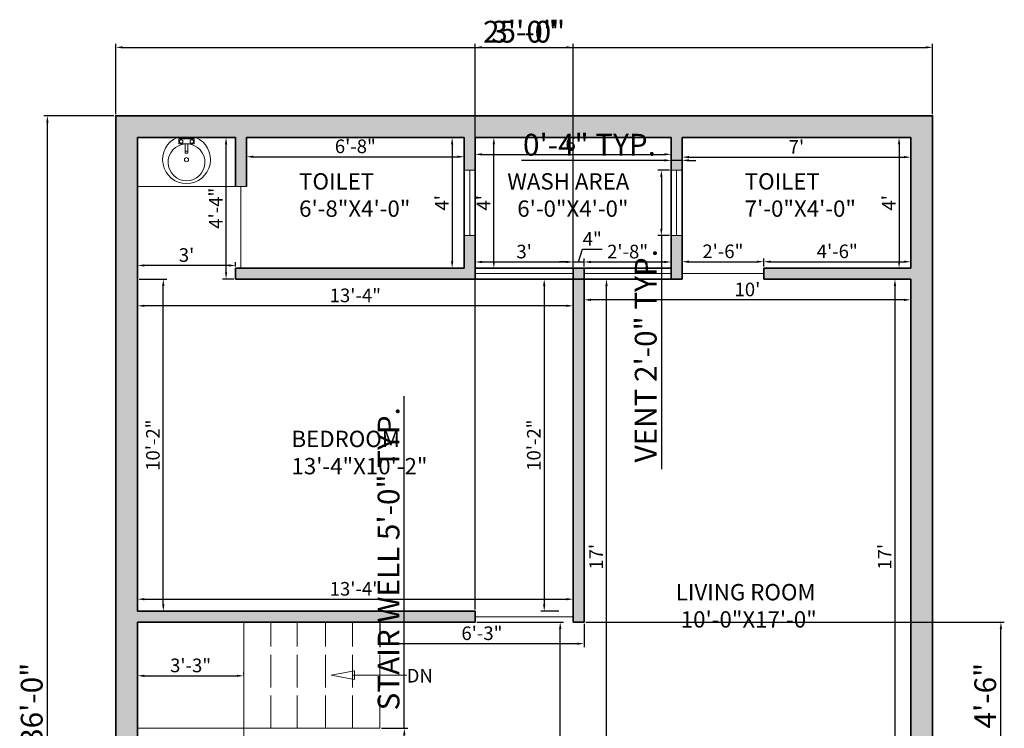
# Model space of a CAD drawing. Units: inches. Extents: x 3259 to 4981, y 1402 to 2026.
# Tile 11 of 11: x 4620 to 4981, y 1682 to 1942. Entities that reach past the tile are written whole.
import ezdxf

# ---------------------------------------------------------------- set-up
doc = ezdxf.new("R2010")
doc.units = ezdxf.units.IN
doc.linetypes.add('ACAD_ISO02W100', pattern=[15, 12, -3])
for name, color, linetype, lineweight in [('A-ANNO-DIMS', 2, 'Continuous', 13), ('A-ANNO-SYMB', 7, 'Continuous', 13), ('A-AREA-IDEN', 7, 'Continuous', 18), ('A-DOOR', 3, 'Continuous', 18), ('A-FLOR-CASE', 8, 'Continuous', 18), ('A-FLOR-FIXT', 9, 'Continuous', 18), ('A-FLOR-STRS', 7, 'Continuous', 18), ('A-FLOR-STRS-OVHD', 8, 'ACAD_ISO02W100', 13), ('A-GLAZ', 4, 'Continuous', 18), ('A-WALL', 7, 'Continuous', 35), ('A-WALL-PATT', 252, 'Continuous', 13)]:
    doc.layers.add(name, color=color, linetype=linetype, lineweight=lineweight)
doc.styles.get("Standard").update_dxf_attribs({"font": 'arial.ttf'})
doc.dimstyles.new('ISO-25', dxfattribs={"dimtxt": 8, "dimasz": 2.5, "dimexe": 1.25, "dimexo": 0.625, "dimtad": 1, "dimdec": 1, "dimlunit": 3, "dimtxsty": 'Standard', "dimcen": 2.5, "dimclrd": 4, "dimclre": 4, "dimclrt": 1, "dimadec": 0, "dimazin": 0, "dimtfac": 1, "dimtdec": 1, "dimtmove": 0, "dimatfit": 3, "dimfxl": 1, "dimarcsym": 0})

# ---------------------------------------------------------------- blocks, each defined once
blk = doc.blocks.new('M_BATH_BASIN_Basin - Oval_P')
at = {"color": 0, "linetype": 'ByBlock', "lineweight": -2}
blk.add_lwpolyline([(0, 89.5, -5.027337), (0, -89.5)], format="xyb", close=True, dxfattribs=at)
blk.add_lwpolyline([(63.2, 12, -30), (63.2, -12, -1.097889)], format="xyb", dxfattribs=at)
for points in [[(13.2, -76.2), (13.2, 76.2), (63.2, 76.2), (63.2, -76.2)], [(19.1, 50.8), (28.7, 67.3), (47.7, 67.3), (57.2, 50.8), (47.7, 34.3), (28.7, 34.3)]]:
    blk.add_lwpolyline(points, close=True, dxfattribs=at)
for points in [[(63.2, 12), (151.6, 12), (151.6, -12), (63.2, -12)], [(134.3, 12), (134.3, -12)], [(28.7, -34.3), (47.7, -34.3), (57.2, -50.8), (47.7, -67.3), (28.7, -67.3), (19.1, -50.8), (28.7, -34.3)]]:
    blk.add_lwpolyline(points, dxfattribs=at)
blk.add_circle((216.2, 0), 20.1, dxfattribs=at)
at = {"layer": 'Defpoints'}
for p in [(0, 234), (0, -234)]:
    blk.add_point(p, dxfattribs=at)
blk = doc.blocks.new('*D71')
at = {"layer": 'A-ANNO-DIMS', "color": 0, "lineweight": -2, "transparency": 16777216}
for p, q in [((4702.83, 1898.49), (4702.83, 1890.79)), ((4782.83, 1898.49), (4782.83, 1890.79)), ((4705.33, 1892.04), (4780.33, 1892.04))]:
    blk.add_line(p, q, dxfattribs=at)
at = {"layer": 'A-ANNO-DIMS', "color": 0, "transparency": 16777216}
for points in [[(4705.33, 1892.46), (4705.33, 1891.63), (4702.83, 1892.04)], [(4780.33, 1892.46), (4780.33, 1891.63), (4782.83, 1892.04)]]:
    blk.add_solid(points, dxfattribs=at)
at = {"layer": 'Defpoints', "color": 0, "transparency": 16777216}
for p in [(4702.83, 1899.12), (4782.83, 1899.12), (4782.83, 1892.04)]:
    blk.add_point(p, dxfattribs=at)
at = {"layer": 'A-ANNO-DIMS', "color": 0, "transparency": 16777216, "insert": (4742.83, 1895.22), "char_height": 5, "attachment_point": 5}
blk.add_mtext('6\'-8"', dxfattribs=at)
blk = doc.blocks.new('*D72')
at = {"layer": 'A-ANNO-DIMS', "color": 0, "lineweight": -2, "transparency": 16777216}
for p, q in [((4782.2, 1899.12), (4777.14, 1899.12)), ((4778.39, 1896.62), (4778.39, 1853.62)), ((4782.2, 1851.12), (4777.14, 1851.12))]:
    blk.add_line(p, q, dxfattribs=at)
at = {"layer": 'A-ANNO-DIMS', "color": 0, "transparency": 16777216}
for points in [[(4777.97, 1896.62), (4778.8, 1896.62), (4778.39, 1899.12)], [(4777.97, 1853.62), (4778.8, 1853.62), (4778.39, 1851.12)]]:
    blk.add_solid(points, dxfattribs=at)
at = {"layer": 'Defpoints', "color": 0, "transparency": 16777216}
for p in [(4782.83, 1899.12), (4778.39, 1851.12), (4782.83, 1851.12)]:
    blk.add_point(p, dxfattribs=at)
at = {"layer": 'A-ANNO-DIMS', "color": 0, "transparency": 16777216, "insert": (4775.26, 1875.12), "char_height": 5, "attachment_point": 5, "rotation": 90}
blk.add_mtext("4'", dxfattribs=at)
blk = doc.blocks.new('*D73')
at = {"layer": 'A-ANNO-DIMS', "color": 0, "lineweight": -2, "transparency": 16777216}
for p, q in [((4787.45, 1899.12), (4794.95, 1899.12)), ((4793.7, 1853.62), (4793.7, 1896.62)), ((4787.45, 1851.12), (4794.95, 1851.12))]:
    blk.add_line(p, q, dxfattribs=at)
at = {"layer": 'A-ANNO-DIMS', "color": 0, "transparency": 16777216}
for points in [[(4793.28, 1896.62), (4794.12, 1896.62), (4793.7, 1899.12)], [(4793.28, 1853.62), (4794.12, 1853.62), (4793.7, 1851.12)]]:
    blk.add_solid(points, dxfattribs=at)
at = {"layer": 'Defpoints', "color": 0, "transparency": 16777216}
for p in [(4786.83, 1899.12), (4793.7, 1899.12), (4786.83, 1851.12)]:
    blk.add_point(p, dxfattribs=at)
at = {"layer": 'A-ANNO-DIMS', "color": 0, "transparency": 16777216, "insert": (4790.57, 1875.12), "char_height": 5, "attachment_point": 5, "rotation": 90}
blk.add_mtext("4'", dxfattribs=at)
blk = doc.blocks.new('*D95')
at = {"layer": 'A-ANNO-DIMS', "color": 0, "lineweight": -2, "transparency": 16777216}
for p, q in [((4786.83, 1898.49), (4786.83, 1891.66)), ((4858.83, 1898.49), (4858.83, 1891.66)), ((4789.33, 1892.91), (4856.33, 1892.91))]:
    blk.add_line(p, q, dxfattribs=at)
at = {"layer": 'A-ANNO-DIMS', "color": 0, "transparency": 16777216}
for points in [[(4789.33, 1893.33), (4789.33, 1892.5), (4786.83, 1892.91)], [(4856.33, 1893.33), (4856.33, 1892.5), (4858.83, 1892.91)]]:
    blk.add_solid(points, dxfattribs=at)
at = {"layer": 'Defpoints', "color": 0, "transparency": 16777216}
for p in [(4786.83, 1899.12), (4858.83, 1899.12), (4858.83, 1892.91)]:
    blk.add_point(p, dxfattribs=at)
at = {"layer": 'A-ANNO-DIMS', "color": 0, "transparency": 16777216, "insert": (4822.83, 1896.09), "char_height": 5, "attachment_point": 5}
blk.add_mtext("6'", dxfattribs=at)
blk = doc.blocks.new('*D96')
at = {"layer": 'A-ANNO-DIMS', "color": 0, "lineweight": -2, "transparency": 16777216}
for p, q in [((4862.83, 1898.49), (4862.83, 1890.65)), ((4946.83, 1898.49), (4946.83, 1890.65)), ((4865.33, 1891.9), (4944.33, 1891.9))]:
    blk.add_line(p, q, dxfattribs=at)
at = {"layer": 'A-ANNO-DIMS', "color": 0, "transparency": 16777216}
for points in [[(4865.33, 1892.31), (4865.33, 1891.48), (4862.83, 1891.9)], [(4944.33, 1892.31), (4944.33, 1891.48), (4946.83, 1891.9)]]:
    blk.add_solid(points, dxfattribs=at)
at = {"layer": 'Defpoints', "color": 0, "transparency": 16777216}
for p in [(4862.83, 1899.12), (4946.83, 1899.12), (4946.83, 1891.9)]:
    blk.add_point(p, dxfattribs=at)
at = {"layer": 'A-ANNO-DIMS', "color": 0, "transparency": 16777216, "insert": (4904.83, 1895.02), "char_height": 5, "attachment_point": 5}
blk.add_mtext("7'", dxfattribs=at)
blk = doc.blocks.new('*D97')
at = {"layer": 'A-ANNO-DIMS', "color": 0, "lineweight": -2, "transparency": 16777216}
for p, q in [((4946.2, 1899.12), (4941.29, 1899.12)), ((4942.54, 1896.62), (4942.54, 1853.62)), ((4946.2, 1851.12), (4941.29, 1851.12))]:
    blk.add_line(p, q, dxfattribs=at)
at = {"layer": 'A-ANNO-DIMS', "color": 0, "transparency": 16777216}
for points in [[(4942.13, 1896.62), (4942.96, 1896.62), (4942.54, 1899.12)], [(4942.13, 1853.62), (4942.96, 1853.62), (4942.54, 1851.12)]]:
    blk.add_solid(points, dxfattribs=at)
at = {"layer": 'Defpoints', "color": 0, "transparency": 16777216}
for p in [(4946.83, 1899.12), (4942.54, 1851.12), (4946.83, 1851.12)]:
    blk.add_point(p, dxfattribs=at)
at = {"layer": 'A-ANNO-DIMS', "color": 0, "transparency": 16777216, "insert": (4939.42, 1875.12), "char_height": 5, "attachment_point": 5, "rotation": 90}
blk.add_mtext("4'", dxfattribs=at)
blk = doc.blocks.new('*D86')
at = {"layer": 'A-ANNO-DIMS', "color": 0, "lineweight": -2, "transparency": 16777216}
for p, q in [((4787.45, 1721.12), (4819.32, 1721.12)), ((4818.07, 1585.62), (4818.07, 1718.62)), ((4822.2, 1583.12), (4816.82, 1583.12))]:
    blk.add_line(p, q, dxfattribs=at)
at = {"layer": 'A-ANNO-DIMS', "color": 0, "transparency": 16777216}
for points in [[(4817.66, 1718.62), (4818.49, 1718.62), (4818.07, 1721.12)], [(4817.66, 1585.62), (4818.49, 1585.62), (4818.07, 1583.12)]]:
    blk.add_solid(points, dxfattribs=at)
at = {"layer": 'Defpoints', "color": 0, "transparency": 16777216}
for p in [(4786.83, 1721.12), (4818.07, 1721.12), (4822.83, 1583.12)]:
    blk.add_point(p, dxfattribs=at)
at = {"layer": 'A-ANNO-DIMS', "color": 0, "transparency": 16777216, "insert": (4814.9, 1652.12), "char_height": 5, "attachment_point": 5, "rotation": 90}
blk.add_mtext('11\'-6"', dxfattribs=at)
blk = doc.blocks.new('*D88')
at = {"layer": 'A-ANNO-DIMS', "color": 0, "lineweight": -2, "transparency": 16777216}
for p, q in [((4827.45, 1847.12), (4836.33, 1847.12)), ((4835.08, 1645.62), (4835.08, 1844.62)), ((4827.45, 1643.12), (4836.33, 1643.12))]:
    blk.add_line(p, q, dxfattribs=at)
at = {"layer": 'A-ANNO-DIMS', "color": 0, "transparency": 16777216}
for points in [[(4834.66, 1844.62), (4835.49, 1844.62), (4835.08, 1847.12)], [(4834.66, 1645.62), (4835.49, 1645.62), (4835.08, 1643.12)]]:
    blk.add_solid(points, dxfattribs=at)
at = {"layer": 'Defpoints', "color": 0, "transparency": 16777216}
for p in [(4826.83, 1847.12), (4835.08, 1847.12), (4826.83, 1643.12)]:
    blk.add_point(p, dxfattribs=at)
at = {"layer": 'A-ANNO-DIMS', "color": 0, "transparency": 16777216, "insert": (4831.94, 1745.12), "char_height": 5, "attachment_point": 5, "rotation": 90}
blk.add_mtext("17'", dxfattribs=at)
blk = doc.blocks.new('*D89')
at = {"layer": 'A-ANNO-DIMS', "color": 0, "lineweight": -2, "transparency": 16777216}
for p, q in [((4662.83, 1702.02), (4662.83, 1702.65)), ((4665.33, 1701.4), (4699.33, 1701.4)), ((4701.83, 1702.02), (4701.83, 1702.65))]:
    blk.add_line(p, q, dxfattribs=at)
at = {"layer": 'A-ANNO-DIMS', "color": 0, "transparency": 16777216}
for points in [[(4665.33, 1701.81), (4665.33, 1700.98), (4662.83, 1701.4)], [(4699.33, 1701.81), (4699.33, 1700.98), (4701.83, 1701.4)]]:
    blk.add_solid(points, dxfattribs=at)
at = {"layer": 'Defpoints', "color": 0, "transparency": 16777216}
for p in [(4662.83, 1701.4), (4701.83, 1701.4), (4701.83, 1701.4)]:
    blk.add_point(p, dxfattribs=at)
at = {"layer": 'A-ANNO-DIMS', "color": 0, "transparency": 16777216, "insert": (4682.33, 1704.57), "char_height": 5, "attachment_point": 5}
blk.add_mtext('3\'-3"', dxfattribs=at)
blk = doc.blocks.new('*D98')
at = {"layer": 'A-ANNO-DIMS', "color": 0, "lineweight": -2, "transparency": 16777216}
for p, q in [((4826.83, 1848.49), (4826.83, 1838.23)), ((4946.83, 1846.49), (4946.83, 1838.23)), ((4944.33, 1839.48), (4829.33, 1839.48))]:
    blk.add_line(p, q, dxfattribs=at)
at = {"layer": 'A-ANNO-DIMS', "color": 0, "transparency": 16777216}
for points in [[(4829.33, 1839.9), (4829.33, 1839.07), (4826.83, 1839.48)], [(4944.33, 1839.9), (4944.33, 1839.07), (4946.83, 1839.48)]]:
    blk.add_solid(points, dxfattribs=at)
at = {"layer": 'Defpoints', "color": 0, "transparency": 16777216}
for p in [(4826.83, 1849.12), (4946.83, 1847.12), (4826.83, 1839.48)]:
    blk.add_point(p, dxfattribs=at)
at = {"layer": 'A-ANNO-DIMS', "color": 0, "transparency": 16777216, "insert": (4886.83, 1842.66), "char_height": 5, "attachment_point": 5}
blk.add_mtext("10'", dxfattribs=at)
blk = doc.blocks.new('*D99')
at = {"layer": 'A-ANNO-DIMS', "color": 0, "lineweight": -2, "transparency": 16777216}
for p, q in [((4946.2, 1847.12), (4939.77, 1847.12)), ((4941.02, 1844.62), (4941.02, 1645.62)), ((4946.2, 1643.12), (4939.77, 1643.12))]:
    blk.add_line(p, q, dxfattribs=at)
at = {"layer": 'A-ANNO-DIMS', "color": 0, "transparency": 16777216}
for points in [[(4940.61, 1844.62), (4941.44, 1844.62), (4941.02, 1847.12)], [(4940.61, 1645.62), (4941.44, 1645.62), (4941.02, 1643.12)]]:
    blk.add_solid(points, dxfattribs=at)
at = {"layer": 'Defpoints', "color": 0, "transparency": 16777216}
for p in [(4946.83, 1847.12), (4941.02, 1643.12), (4946.83, 1643.12)]:
    blk.add_point(p, dxfattribs=at)
at = {"layer": 'A-ANNO-DIMS', "color": 0, "transparency": 16777216, "insert": (4937.89, 1745.12), "char_height": 5, "attachment_point": 5, "rotation": 90}
blk.add_mtext("17'", dxfattribs=at)
blk = doc.blocks.new('*D100')
at = {"layer": 'A-ANNO-DIMS', "color": 0, "lineweight": -2, "transparency": 16777216}
for p, q in [((4662.83, 1846.49), (4662.83, 1836.05)), ((4822.83, 1846.49), (4822.83, 1836.05)), ((4820.33, 1837.3), (4665.33, 1837.3))]:
    blk.add_line(p, q, dxfattribs=at)
at = {"layer": 'A-ANNO-DIMS', "color": 0, "transparency": 16777216}
for points in [[(4665.33, 1837.71), (4665.33, 1836.88), (4662.83, 1837.3)], [(4820.33, 1837.71), (4820.33, 1836.88), (4822.83, 1837.3)]]:
    blk.add_solid(points, dxfattribs=at)
at = {"layer": 'Defpoints', "color": 0, "transparency": 16777216}
for p in [(4662.83, 1847.12), (4822.83, 1847.12), (4662.83, 1837.3)]:
    blk.add_point(p, dxfattribs=at)
at = {"layer": 'A-ANNO-DIMS', "color": 0, "transparency": 16777216, "insert": (4742.83, 1840.48), "char_height": 5, "attachment_point": 5}
blk.add_mtext('13\'-4"', dxfattribs=at)
blk = doc.blocks.new('*D101')
at = {"layer": 'A-ANNO-DIMS', "color": 0, "lineweight": -2, "transparency": 16777216}
for p, q in [((4662.83, 1725.74), (4662.83, 1730.78)), ((4665.33, 1729.53), (4820.33, 1729.53)), ((4822.83, 1725.74), (4822.83, 1730.78))]:
    blk.add_line(p, q, dxfattribs=at)
at = {"layer": 'A-ANNO-DIMS', "color": 0, "transparency": 16777216}
for points in [[(4665.33, 1729.95), (4665.33, 1729.12), (4662.83, 1729.53)], [(4820.33, 1729.95), (4820.33, 1729.12), (4822.83, 1729.53)]]:
    blk.add_solid(points, dxfattribs=at)
at = {"layer": 'Defpoints', "color": 0, "transparency": 16777216}
for p in [(4822.83, 1729.53), (4662.83, 1725.12), (4822.83, 1725.12)]:
    blk.add_point(p, dxfattribs=at)
at = {"layer": 'A-ANNO-DIMS', "color": 0, "transparency": 16777216, "insert": (4742.83, 1732.71), "char_height": 5, "attachment_point": 5}
blk.add_mtext('13\'-4"', dxfattribs=at)
blk = doc.blocks.new('*D102')
at = {"layer": 'A-ANNO-DIMS', "color": 0, "lineweight": -2, "transparency": 16777216}
for p, q in [((4663.45, 1847.12), (4673.56, 1847.12)), ((4672.31, 1727.62), (4672.31, 1844.62)), ((4663.45, 1725.12), (4673.56, 1725.12))]:
    blk.add_line(p, q, dxfattribs=at)
at = {"layer": 'A-ANNO-DIMS', "color": 0, "transparency": 16777216}
for points in [[(4671.9, 1844.62), (4672.73, 1844.62), (4672.31, 1847.12)], [(4671.9, 1727.62), (4672.73, 1727.62), (4672.31, 1725.12)]]:
    blk.add_solid(points, dxfattribs=at)
at = {"layer": 'Defpoints', "color": 0, "transparency": 16777216}
for p in [(4662.83, 1847.12), (4672.31, 1847.12), (4662.83, 1725.12)]:
    blk.add_point(p, dxfattribs=at)
at = {"layer": 'A-ANNO-DIMS', "color": 0, "transparency": 16777216, "insert": (4669.13, 1786.12), "char_height": 5, "attachment_point": 5, "rotation": 90}
blk.add_mtext('10\'-2"', dxfattribs=at)
blk = doc.blocks.new('*D103')
at = {"layer": 'A-ANNO-DIMS', "color": 0, "lineweight": -2, "transparency": 16777216}
for p, q in [((4817.52, 1847.12), (4810.96, 1847.12)), ((4812.21, 1844.62), (4812.21, 1727.62)), ((4817.52, 1725.12), (4810.96, 1725.12))]:
    blk.add_line(p, q, dxfattribs=at)
at = {"layer": 'A-ANNO-DIMS', "color": 0, "transparency": 16777216}
for points in [[(4811.79, 1844.62), (4812.62, 1844.62), (4812.21, 1847.12)], [(4811.79, 1727.62), (4812.62, 1727.62), (4812.21, 1725.12)]]:
    blk.add_solid(points, dxfattribs=at)
at = {"layer": 'Defpoints', "color": 0, "transparency": 16777216}
for p in [(4818.15, 1847.12), (4812.21, 1725.12), (4818.15, 1725.12)]:
    blk.add_point(p, dxfattribs=at)
at = {"layer": 'A-ANNO-DIMS', "color": 0, "transparency": 16777216, "insert": (4809.03, 1786.12), "char_height": 5, "attachment_point": 5, "rotation": 90}
blk.add_mtext('10\'-2"', dxfattribs=at)
blk = doc.blocks.new('*D104')
at = {"layer": 'A-ANNO-DIMS', "color": 0, "lineweight": -2, "transparency": 16777216}
for p, q in [((4662.83, 1851.74), (4662.83, 1853.36)), ((4696.33, 1852.11), (4665.33, 1852.11)), ((4698.83, 1851.74), (4698.83, 1853.36))]:
    blk.add_line(p, q, dxfattribs=at)
at = {"layer": 'A-ANNO-DIMS', "color": 0, "transparency": 16777216}
for points in [[(4665.33, 1852.52), (4665.33, 1851.69), (4662.83, 1852.11)], [(4696.33, 1852.52), (4696.33, 1851.69), (4698.83, 1852.11)]]:
    blk.add_solid(points, dxfattribs=at)
at = {"layer": 'Defpoints', "color": 0, "transparency": 16777216}
for p in [(4662.83, 1852.11), (4662.83, 1851.12), (4698.83, 1851.12)]:
    blk.add_point(p, dxfattribs=at)
at = {"layer": 'A-ANNO-DIMS', "color": 0, "transparency": 16777216, "insert": (4680.83, 1855.29), "char_height": 5, "attachment_point": 5}
blk.add_mtext("3'", dxfattribs=at)
blk = doc.blocks.new('*D105')
at = {"layer": 'A-ANNO-DIMS', "color": 0, "lineweight": -2, "transparency": 16777216}
for p, q in [((4698.2, 1899.12), (4694.11, 1899.12)), ((4695.36, 1849.62), (4695.36, 1896.62)), ((4698.2, 1847.12), (4694.11, 1847.12))]:
    blk.add_line(p, q, dxfattribs=at)
at = {"layer": 'A-ANNO-DIMS', "color": 0, "transparency": 16777216}
for points in [[(4694.95, 1896.62), (4695.78, 1896.62), (4695.36, 1899.12)], [(4694.95, 1849.62), (4695.78, 1849.62), (4695.36, 1847.12)]]:
    blk.add_solid(points, dxfattribs=at)
at = {"layer": 'Defpoints', "color": 0, "transparency": 16777216}
for p in [(4695.36, 1899.12), (4698.83, 1899.12), (4698.83, 1847.12)]:
    blk.add_point(p, dxfattribs=at)
at = {"layer": 'A-ANNO-DIMS', "color": 0, "transparency": 16777216, "insert": (4692.24, 1873.12), "char_height": 5, "attachment_point": 5, "rotation": 90}
blk.add_mtext('4\'-4"', dxfattribs=at)
blk = doc.blocks.new('*D106')
at = {"layer": 'A-ANNO-DIMS', "color": 0, "lineweight": -2, "transparency": 16777216}
for p, q in [((4751.83, 1720.49), (4751.83, 1711.96)), ((4826.83, 1720.49), (4826.83, 1711.96)), ((4754.33, 1713.21), (4824.33, 1713.21))]:
    blk.add_line(p, q, dxfattribs=at)
at = {"layer": 'A-ANNO-DIMS', "color": 0, "transparency": 16777216}
for points in [[(4754.33, 1713.63), (4754.33, 1712.8), (4751.83, 1713.21)], [(4824.33, 1713.63), (4824.33, 1712.8), (4826.83, 1713.21)]]:
    blk.add_solid(points, dxfattribs=at)
at = {"layer": 'Defpoints', "color": 0, "transparency": 16777216}
for p in [(4751.83, 1721.12), (4826.83, 1721.12), (4826.83, 1713.21)]:
    blk.add_point(p, dxfattribs=at)
at = {"layer": 'A-ANNO-DIMS', "color": 0, "transparency": 16777216, "insert": (4789.33, 1716.39), "char_height": 5, "attachment_point": 5}
blk.add_mtext('6\'-3"', dxfattribs=at)
blk = doc.blocks.new('*D127')
at = {"layer": 'A-ANNO-DIMS', "color": 0, "lineweight": -2, "transparency": 16777216}
for p, q in [((4786.83, 1851.74), (4786.83, 1854.64)), ((4789.33, 1853.39), (4820.33, 1853.39)), ((4822.83, 1851.74), (4822.83, 1854.64))]:
    blk.add_line(p, q, dxfattribs=at)
at = {"layer": 'A-ANNO-DIMS', "color": 0, "transparency": 16777216}
for points in [[(4789.33, 1853.81), (4789.33, 1852.97), (4786.83, 1853.39)], [(4820.33, 1853.81), (4820.33, 1852.97), (4822.83, 1853.39)]]:
    blk.add_solid(points, dxfattribs=at)
at = {"layer": 'Defpoints', "color": 0, "transparency": 16777216}
for p in [(4822.83, 1853.39), (4786.83, 1851.12), (4822.83, 1851.12)]:
    blk.add_point(p, dxfattribs=at)
at = {"layer": 'A-ANNO-DIMS', "color": 0, "transparency": 16777216, "insert": (4804.83, 1856.57), "char_height": 5, "attachment_point": 5}
blk.add_mtext("3'", dxfattribs=at)
blk = doc.blocks.new('*D128')
at = {"layer": 'A-ANNO-DIMS', "color": 0, "lineweight": -2, "transparency": 16777216}
for p, q in [((4824.83, 1853.39), (4826.24, 1858.08)), ((4826.24, 1858.08), (4833.43, 1858.08)), ((4820.33, 1853.39), (4817.83, 1853.39)), ((4822.83, 1851.74), (4822.83, 1854.64)), ((4822.83, 1853.39), (4826.83, 1853.39)), ((4822.83, 1853.39), (4826.83, 1853.39)), ((4826.83, 1851.74), (4826.83, 1854.64)), ((4829.33, 1853.39), (4831.83, 1853.39))]:
    blk.add_line(p, q, dxfattribs=at)
at = {"layer": 'A-ANNO-DIMS', "color": 0, "transparency": 16777216}
for points in [[(4820.33, 1853.81), (4820.33, 1852.97), (4822.83, 1853.39)], [(4829.33, 1853.81), (4829.33, 1852.97), (4826.83, 1853.39)]]:
    blk.add_solid(points, dxfattribs=at)
at = {"layer": 'Defpoints', "color": 0, "transparency": 16777216}
for p in [(4826.83, 1853.39), (4822.83, 1851.12), (4826.83, 1851.12)]:
    blk.add_point(p, dxfattribs=at)
at = {"layer": 'A-ANNO-DIMS', "color": 0, "transparency": 16777216, "insert": (4829.84, 1861.2), "char_height": 5, "attachment_point": 5}
blk.add_mtext('4"', dxfattribs=at)
blk = doc.blocks.new('*D129')
at = {"layer": 'A-ANNO-DIMS', "color": 0, "lineweight": -2, "transparency": 16777216}
for p, q in [((4826.83, 1851.74), (4826.83, 1854.64)), ((4829.33, 1853.39), (4856.33, 1853.39)), ((4858.83, 1851.74), (4858.83, 1854.64))]:
    blk.add_line(p, q, dxfattribs=at)
at = {"layer": 'A-ANNO-DIMS', "color": 0, "transparency": 16777216}
for points in [[(4829.33, 1853.81), (4829.33, 1852.97), (4826.83, 1853.39)], [(4856.33, 1853.81), (4856.33, 1852.97), (4858.83, 1853.39)]]:
    blk.add_solid(points, dxfattribs=at)
at = {"layer": 'Defpoints', "color": 0, "transparency": 16777216}
for p in [(4858.83, 1853.39), (4826.83, 1851.12), (4858.83, 1851.12)]:
    blk.add_point(p, dxfattribs=at)
at = {"layer": 'A-ANNO-DIMS', "color": 0, "transparency": 16777216, "insert": (4842.83, 1856.57), "char_height": 5, "attachment_point": 5}
blk.add_mtext('2\'-8"', dxfattribs=at)
blk = doc.blocks.new('*D130')
at = {"layer": 'A-ANNO-DIMS', "color": 0, "lineweight": -2, "transparency": 16777216}
for p, q in [((4862.83, 1854.02), (4862.83, 1854.73)), ((4865.33, 1853.48), (4890.33, 1853.48)), ((4892.83, 1851.74), (4892.83, 1854.73))]:
    blk.add_line(p, q, dxfattribs=at)
at = {"layer": 'A-ANNO-DIMS', "color": 0, "transparency": 16777216}
for points in [[(4865.33, 1853.9), (4865.33, 1853.07), (4862.83, 1853.48)], [(4890.33, 1853.9), (4890.33, 1853.07), (4892.83, 1853.48)]]:
    blk.add_solid(points, dxfattribs=at)
at = {"layer": 'Defpoints', "color": 0, "transparency": 16777216}
for p in [(4862.83, 1853.39), (4892.83, 1853.48), (4892.83, 1851.12)]:
    blk.add_point(p, dxfattribs=at)
at = {"layer": 'A-ANNO-DIMS', "color": 0, "transparency": 16777216, "insert": (4877.83, 1856.66), "char_height": 5, "attachment_point": 5}
blk.add_mtext('2\'-6"', dxfattribs=at)
blk = doc.blocks.new('*D131')
at = {"layer": 'A-ANNO-DIMS', "color": 0, "lineweight": -2, "transparency": 16777216}
for p, q in [((4892.83, 1851.74), (4892.83, 1854.73)), ((4895.33, 1853.48), (4944.33, 1853.48)), ((4946.83, 1854.11), (4946.83, 1854.73))]:
    blk.add_line(p, q, dxfattribs=at)
at = {"layer": 'A-ANNO-DIMS', "color": 0, "transparency": 16777216}
for points in [[(4895.33, 1853.9), (4895.33, 1853.07), (4892.83, 1853.48)], [(4944.33, 1853.9), (4944.33, 1853.07), (4946.83, 1853.48)]]:
    blk.add_solid(points, dxfattribs=at)
at = {"layer": 'Defpoints', "color": 0, "transparency": 16777216}
for p in [(4946.83, 1853.48), (4946.83, 1853.48), (4892.83, 1851.12)]:
    blk.add_point(p, dxfattribs=at)
at = {"layer": 'A-ANNO-DIMS', "color": 0, "transparency": 16777216, "insert": (4919.83, 1856.66), "char_height": 5, "attachment_point": 5}
blk.add_mtext('4\'-6"', dxfattribs=at)
blk = doc.blocks.new('VENT-24x4')
for p, q in [((0, 24), (4, 24)), ((2, 24), (2, 0)), ((0, 0), (4, 0))]:
    blk.add_line(p, q)
blk = doc.blocks.new('STAIR-DIRECTION')
blk.add_line((7.93, 1.55), (27.85, 1.55))
blk.add_lwpolyline([(0, 1.55), (8.64, 3.11), (8.64, 0)], close=True)
blk = doc.blocks.new('*D146')
at = {"layer": 'A-ANNO-DIMS', "color": 4, "lineweight": -2, "transparency": 16777216}
for p, q in [((4858.2, 1887.12), (4853.98, 1887.12)), ((4855.23, 1884.62), (4855.23, 1865.62)), ((4858.2, 1863.12), (4853.98, 1863.12)), ((4855.23, 1863.12), (4855.23, 1777.28))]:
    blk.add_line(p, q, dxfattribs=at)
at = {"layer": 'A-ANNO-DIMS', "color": 4, "transparency": 16777216}
for points in [[(4854.81, 1884.62), (4855.65, 1884.62), (4855.23, 1887.12)], [(4854.81, 1865.62), (4855.65, 1865.62), (4855.23, 1863.12)]]:
    blk.add_solid(points, dxfattribs=at)
at = {"layer": 'Defpoints', "color": 0, "transparency": 16777216}
for p in [(4858.83, 1887.12), (4855.23, 1863.12), (4858.83, 1863.12)]:
    blk.add_point(p, dxfattribs=at)
at = {"layer": 'A-ANNO-DIMS', "color": 1, "transparency": 16777216, "insert": (4850.52, 1818.95), "char_height": 8, "attachment_point": 5, "rotation": 90}
blk.add_mtext('VENT 2\'-0" TYP.', dxfattribs=at)
blk = doc.blocks.new('*D147')
at = {"layer": 'A-ANNO-DIMS', "color": 4, "lineweight": -2, "transparency": 16777216}
for p, q in [((4858.83, 1887.74), (4858.83, 1891.97)), ((4862.83, 1887.74), (4862.83, 1891.97)), ((4856.33, 1890.72), (4803.82, 1890.72)), ((4862.83, 1890.72), (4858.83, 1890.72)), ((4865.33, 1890.72), (4867.83, 1890.72))]:
    blk.add_line(p, q, dxfattribs=at)
at = {"layer": 'A-ANNO-DIMS', "color": 4, "transparency": 16777216}
for points in [[(4856.33, 1891.13), (4856.33, 1890.3), (4858.83, 1890.72)], [(4865.33, 1891.13), (4865.33, 1890.3), (4862.83, 1890.72)]]:
    blk.add_solid(points, dxfattribs=at)
at = {"layer": 'Defpoints', "color": 0, "transparency": 16777216}
for p in [(4858.83, 1890.72), (4858.83, 1887.12), (4862.83, 1887.12)]:
    blk.add_point(p, dxfattribs=at)
at = {"layer": 'A-ANNO-DIMS', "color": 1, "transparency": 16777216, "insert": (4828.82, 1895.43), "char_height": 8, "attachment_point": 5}
blk.add_mtext('0\'-4" TYP.', dxfattribs=at)
blk = doc.blocks.new('*D154')
at = {"layer": 'A-ANNO-DIMS', "color": 4, "lineweight": -2, "transparency": 16777216}
for p, q in [((4760.83, 1682.12), (4760.83, 1804.15)), ((4752.45, 1682.12), (4762.08, 1682.12)), ((4760.83, 1624.62), (4760.83, 1679.62)), ((4752.45, 1622.12), (4762.08, 1622.12))]:
    blk.add_line(p, q, dxfattribs=at)
at = {"layer": 'A-ANNO-DIMS', "color": 4, "transparency": 16777216}
for points in [[(4760.41, 1679.62), (4761.25, 1679.62), (4760.83, 1682.12)], [(4760.41, 1624.62), (4761.25, 1624.62), (4760.83, 1622.12)]]:
    blk.add_solid(points, dxfattribs=at)
at = {"layer": 'Defpoints', "color": 0, "transparency": 16777216}
for p in [(4751.83, 1682.12), (4760.83, 1682.12), (4751.83, 1622.12)]:
    blk.add_point(p, dxfattribs=at)
at = {"layer": 'A-ANNO-DIMS', "color": 1, "transparency": 16777216, "insert": (4756.07, 1744.38), "char_height": 8, "attachment_point": 5, "rotation": 90}
blk.add_mtext('STAIR WELL 5\'-0" TYP.', dxfattribs=at)
blk = doc.blocks.new('*D188')
at = {"layer": 'A-ANNO-DIMS', "color": 4, "lineweight": -2, "transparency": 16777216}
for p, q in [((4654.83, 1907.74), (4654.83, 1933.47)), ((4657.33, 1932.22), (4952.33, 1932.22)), ((4954.83, 1907.74), (4954.83, 1933.47))]:
    blk.add_line(p, q, dxfattribs=at)
at = {"layer": 'A-ANNO-DIMS', "color": 4, "transparency": 16777216}
for points in [[(4657.33, 1932.63), (4657.33, 1931.8), (4654.83, 1932.22)], [(4952.33, 1932.63), (4952.33, 1931.8), (4954.83, 1932.22)]]:
    blk.add_solid(points, dxfattribs=at)
at = {"layer": 'Defpoints', "color": 0, "transparency": 16777216}
for p in [(4954.83, 1932.22), (4654.83, 1907.12), (4954.83, 1907.12)]:
    blk.add_point(p, dxfattribs=at)
at = {"layer": 'A-ANNO-DIMS', "color": 1, "transparency": 16777216, "insert": (4804.83, 1936.93), "char_height": 8, "attachment_point": 5}
blk.add_mtext('25\'-0"', dxfattribs=at)
blk = doc.blocks.new('*D189')
at = {"layer": 'A-ANNO-DIMS', "color": 4, "lineweight": -2, "transparency": 16777216}
for p, q in [((4654.2, 1907.12), (4628.48, 1907.12)), ((4629.73, 1477.62), (4629.73, 1904.62)), ((4654.2, 1475.12), (4628.48, 1475.12))]:
    blk.add_line(p, q, dxfattribs=at)
at = {"layer": 'A-ANNO-DIMS', "color": 4, "transparency": 16777216}
for points in [[(4629.31, 1904.62), (4630.15, 1904.62), (4629.73, 1907.12)], [(4629.31, 1477.62), (4630.15, 1477.62), (4629.73, 1475.12)]]:
    blk.add_solid(points, dxfattribs=at)
at = {"layer": 'Defpoints', "color": 0, "transparency": 16777216}
for p in [(4629.73, 1907.12), (4654.83, 1907.12), (4654.83, 1475.12)]:
    blk.add_point(p, dxfattribs=at)
at = {"layer": 'A-ANNO-DIMS', "color": 1, "transparency": 16777216, "insert": (4625.02, 1691.12), "char_height": 8, "attachment_point": 5, "rotation": 90}
blk.add_mtext('36\'-0"', dxfattribs=at)
blk = doc.blocks.new('*D196')
at = {"layer": 'A-ANNO-DIMS', "color": 4, "lineweight": -2, "transparency": 16777216}
for p, q in [((4786.83, 1725.74), (4786.83, 1933.47)), ((4789.33, 1932.22), (4820.33, 1932.22)), ((4822.83, 1723.74), (4822.83, 1933.47))]:
    blk.add_line(p, q, dxfattribs=at)
at = {"layer": 'A-ANNO-DIMS', "color": 4, "transparency": 16777216}
for points in [[(4789.33, 1932.63), (4789.33, 1931.8), (4786.83, 1932.22)], [(4820.33, 1932.63), (4820.33, 1931.8), (4822.83, 1932.22)]]:
    blk.add_solid(points, dxfattribs=at)
at = {"layer": 'Defpoints', "color": 0, "transparency": 16777216}
for p in [(4822.83, 1932.22), (4786.83, 1725.12), (4822.83, 1723.12)]:
    blk.add_point(p, dxfattribs=at)
at = {"layer": 'A-ANNO-DIMS', "color": 1, "transparency": 16777216, "insert": (4804.83, 1936.93), "char_height": 8, "attachment_point": 5}
blk.add_mtext('3\'-0"', dxfattribs=at)
blk = doc.blocks.new('*D197')
at = {"layer": 'A-ANNO-DIMS', "color": 4, "lineweight": -2, "transparency": 16777216}
for p, q in [((4827.45, 1721.12), (4981.18, 1721.12)), ((4979.93, 1669.62), (4979.93, 1718.62)), ((4827.45, 1667.12), (4981.18, 1667.12))]:
    blk.add_line(p, q, dxfattribs=at)
at = {"layer": 'A-ANNO-DIMS', "color": 4, "transparency": 16777216}
for points in [[(4979.51, 1718.62), (4980.35, 1718.62), (4979.93, 1721.12)], [(4979.51, 1669.62), (4980.35, 1669.62), (4979.93, 1667.12)]]:
    blk.add_solid(points, dxfattribs=at)
at = {"layer": 'Defpoints', "color": 0, "transparency": 16777216}
for p in [(4826.83, 1721.12), (4979.93, 1721.12), (4826.83, 1667.12)]:
    blk.add_point(p, dxfattribs=at)
at = {"layer": 'A-ANNO-DIMS', "color": 1, "transparency": 16777216, "insert": (4975.22, 1694.12), "char_height": 8, "attachment_point": 5, "rotation": 90}
blk.add_mtext('4\'-6"', dxfattribs=at)

msp = doc.modelspace()

# ---------------------------------------------------------------- hatches: boundary and pattern name
at = {"layer": 'A-WALL-PATT'}
h = msp.add_hatch(color=256, dxfattribs=at)
h.dxf.hatch_style = 1
h.paths.add_polyline_path([(4826.83, 1851.12), (4822.83, 1851.12), (4822.83, 1721.12), (4826.83, 1721.12), (4826.83, 1777.43), (4826.82, 1777.43), (4826.82, 1777.47), (4826.83, 1777.47), (4826.83, 1781.5), (4826.83, 1781.5), (4826.83, 1781.55)], flags=17)
h.paths.add_polyline_path([(4786.83, 1863.12), (4782.83, 1863.12), (4782.83, 1851.12), (4698.83, 1851.12), (4698.83, 1847.12), (4736.66, 1847.12), (4736.66, 1847.13), (4736.7, 1847.13), (4736.7, 1847.12), (4740.73, 1847.12), (4740.73, 1847.12), (4740.78, 1847.12), (4786.83, 1847.12)], flags=17)
h.paths.add_polyline_path([(4862.83, 1863.12), (4858.83, 1863.12), (4858.83, 1847.12), (4862.83, 1847.12)], flags=17)
h.paths.add_polyline_path([(4954.83, 1907.12), (4654.83, 1907.12), (4654.83, 1579.12), (4826.83, 1579.12), (4826.83, 1587.12), (4822.83, 1587.12), (4822.83, 1583.12), (4662.83, 1583.12), (4662.83, 1721.12), (4786.83, 1721.12), (4786.83, 1725.12), (4662.83, 1725.12), (4662.83, 1899.12), (4698.83, 1899.12), (4698.83, 1881.12), (4702.83, 1881.12), (4702.83, 1899.12), (4782.83, 1899.12), (4782.83, 1887.12), (4786.83, 1887.12), (4786.83, 1899.12), (4858.83, 1899.12), (4858.83, 1887.12), (4862.83, 1887.12), (4862.83, 1899.12), (4946.83, 1899.12), (4946.83, 1851.12), (4892.83, 1851.12), (4892.83, 1847.12), (4946.83, 1847.12), (4946.83, 1643.12), (4928.83, 1643.12), (4928.83, 1639.12), (4954.83, 1639.12)])
h.paths.add_polyline_path([(4826.83, 1667.12), (4822.83, 1667.12), (4822.83, 1635.12), (4826.83, 1635.12), (4826.83, 1639.12), (4844.83, 1639.12), (4844.83, 1643.12), (4826.83, 1643.12)], flags=17)

# ---------------------------------------------------------------- linework, layer by layer
at = {"layer": 'A-DOOR'}
for p, q in [((4700.83, 1881.12), (4700.83, 1851.12)), ((4826.83, 1849.12), (4858.83, 1849.12)), ((4892.83, 1849.12), (4862.83, 1849.12)), ((4786.83, 1723.12), (4822.83, 1723.12))]:
    msp.add_line(p, q, dxfattribs=at)
at = {"layer": 'A-FLOR-CASE'}
msp.add_line((4662.83, 1881.12), (4702.83, 1881.12), dxfattribs=at)
at = {"layer": 'A-FLOR-STRS'}
for p, q in [((4701.83, 1583.12), (4701.83, 1721.12)), ((4662.83, 1682.12), (4751.83, 1682.12))]:
    msp.add_line(p, q, dxfattribs=at)
at = {"layer": 'A-FLOR-STRS-OVHD'}
for p, q in [((4711.83, 1682.12), (4711.83, 1721.12)), ((4721.45, 1682.12), (4721.45, 1721.12)), ((4731.83, 1682.12), (4731.83, 1721.12)), ((4741.83, 1682.12), (4741.83, 1721.12)), ((4751.83, 1682.12), (4751.83, 1721.12))]:
    msp.add_line(p, q, dxfattribs=at)
at = {"layer": 'A-GLAZ'}
msp.add_line((4786.83, 1849.12), (4822.83, 1849.12), dxfattribs=at)
at = {"layer": 'A-WALL'}
for p, q in [((4662.83, 1899.12), (4698.83, 1899.12)), ((4662.83, 1725.12), (4662.83, 1899.12)), ((4698.83, 1899.12), (4698.83, 1881.12)), ((4702.83, 1899.12), (4782.83, 1899.12)), ((4702.83, 1899.12), (4702.83, 1881.12)), ((4782.83, 1899.12), (4782.83, 1851.12)), ((4786.83, 1899.12), (4858.83, 1899.12)), ((4786.83, 1899.12), (4786.83, 1847.12)), ((4858.83, 1899.12), (4858.83, 1847.12)), ((4862.83, 1899.12), (4946.83, 1899.12)), ((4862.83, 1899.12), (4862.83, 1847.12)), ((4946.83, 1899.12), (4946.83, 1851.12)), ((4698.83, 1851.12), (4782.83, 1851.12)), ((4698.83, 1851.12), (4698.83, 1847.12)), ((4786.83, 1851.12), (4858.83, 1851.12)), ((4822.83, 1721.12), (4822.83, 1851.12)), ((4826.83, 1721.12), (4826.83, 1851.12)), ((4892.83, 1851.12), (4946.83, 1851.12)), ((4892.83, 1851.12), (4892.83, 1847.12)), ((4698.83, 1847.12), (4858.83, 1847.12)), ((4858.83, 1847.12), (4862.83, 1847.12)), ((4892.83, 1847.12), (4946.83, 1847.12)), ((4946.83, 1847.12), (4946.83, 1643.12)), ((4662.83, 1725.12), (4786.83, 1725.12)), ((4786.83, 1721.12), (4786.83, 1725.12)), ((4662.83, 1721.12), (4786.83, 1721.12)), ((4662.83, 1583.12), (4662.83, 1721.12)), ((4822.83, 1721.12), (4826.83, 1721.12))]:
    msp.add_line(p, q, dxfattribs=at)
msp.add_lwpolyline([(4946.83, 1475.12), (4654.83, 1475.12), (4654.83, 1907.12), (4954.83, 1907.12), (4954.83, 1475.12), (4946.83, 1475.12)], dxfattribs=at)

# ---------------------------------------------------------------- block references
at = {"layer": 'A-ANNO-SYMB'}
msp.add_blockref('STAIR-DIRECTION', (4733.94, 1700.06), dxfattribs=at)
at = {"layer": 'A-FLOR-FIXT', "xscale": -0.0376189459335944, "yscale": 0.0376189459335944, "zscale": 0.0376189459335944, "rotation": 90}
msp.add_blockref('M_BATH_BASIN_Basin - Oval_P', (4680.83, 1899.12), dxfattribs=at)
at = {"layer": 'A-GLAZ'}
msp.add_blockref('VENT-24x4', (4782.83, 1863.12), dxfattribs=at)
at = {"layer": 'A-GLAZ', "rotation": 180}
msp.add_blockref('VENT-24x4', (4862.83, 1887.12), dxfattribs=at)

# ---------------------------------------------------------------- texts
at = {"layer": 'A-ANNO-SYMB', "insert": (4771.31, 1703.94), "char_height": 5, "attachment_point": 3}
msp.add_mtext_dynamic_manual_height_columns('DN', width=10.7355, gutter_width=12.5, heights=[0], dxfattribs=at)
at = {"layer": 'A-AREA-IDEN', "char_height": 6, "attachment_point": 1}
for s, width, insert in [('TOILET\\P6\'-8"X4\'-0"', 127.3061, (4722.19, 1885.99)), ('WASH AREA\\P  6\'-0"X4\'-0"', 127.3061, (4798.64, 1885.99)), ('TOILET\\P7\'-0"X4\'-0"', 127.3061, (4885.85, 1885.99)), ('BEDROOM\\P13\'-4"X10\'-2"', 86.9528, (4719.39, 1791.41)), ('LIVING ROOM\\P 10\'-0"X17\'-0"', 127.3061, (4860.53, 1735.12))]:
    msp.add_mtext_dynamic_manual_height_columns(s, width=width, gutter_width=12.5, heights=[0], dxfattribs=dict(at, insert=insert))

# ---------------------------------------------------------------- dimensions: what is measured, and where the dimension line sits
at = {"layer": 'A-ANNO-DIMS'}
for base, p1, p2, override, picture, middle in [((4954.83, 1932.22), (4654.83, 1907.12), (4954.83, 1907.12), {"dimdec": 1, "dimlfac": 1, "dimrnd": 0, "dimzin": 1, "dimdsep": 46, "dimlunit": 4, "dimfrac": 2}, '*D188', (4804.83, 1936.93)), ((4822.83, 1932.22), (4786.83, 1725.12), (4822.83, 1723.12), {"dimdec": 1, "dimlfac": 1, "dimrnd": 0, "dimzin": 1, "dimdsep": 46, "dimlunit": 4, "dimfrac": 2}, '*D196', (4804.83, 1936.93)), ((4782.83, 1892.04), (4702.83, 1899.12), (4782.83, 1899.12), {"dimtxt": 5, "dimclrd": 0, "dimclre": 0, "dimclrt": 0}, '*D71', (4742.83, 1895.22)), ((4858.83, 1892.91), (4786.83, 1899.12), (4858.83, 1899.12), {"dimtxt": 5, "dimclrd": 0, "dimclre": 0, "dimclrt": 0}, '*D95', (4822.83, 1896.09)), ((4946.83, 1891.9), (4862.83, 1899.12), (4946.83, 1899.12), {"dimtxt": 5, "dimclrd": 0, "dimclre": 0, "dimclrt": 0}, '*D96', (4904.83, 1895.02)), ((4826.83, 1853.39), (4822.83, 1851.12), (4826.83, 1851.12), {"dimtxt": 5, "dimclrd": 0, "dimclre": 0, "dimclrt": 0, "dimtmove": 1}, '*D128', (4826.86, 1861.2)), ((4822.83, 1853.39), (4786.83, 1851.12), (4822.83, 1851.12), {"dimtxt": 5, "dimclrd": 0, "dimclre": 0, "dimclrt": 0}, '*D127', (4804.83, 1856.57)), ((4858.83, 1853.39), (4826.83, 1851.12), (4858.83, 1851.12), {"dimtxt": 5, "dimclrd": 0, "dimclre": 0, "dimclrt": 0, "dimtmove": 1}, '*D129', (4842.83, 1856.57)), ((4892.83, 1853.48), (4862.83, 1853.39), (4892.83, 1851.12), {"dimtxt": 5, "dimclrd": 0, "dimclre": 0, "dimclrt": 0}, '*D130', (4877.83, 1856.66)), ((4946.83, 1853.48), (4892.83, 1851.12), (4946.83, 1853.48), {"dimtxt": 5, "dimclrd": 0, "dimclre": 0, "dimclrt": 0, "dimtmove": 1}, '*D131', (4919.83, 1856.66)), ((4662.83, 1852.11), (4698.83, 1851.12), (4662.83, 1851.12), {"dimtxt": 5, "dimclrd": 0, "dimclre": 0, "dimclrt": 0}, '*D104', (4680.83, 1855.29)), ((4826.83, 1839.48), (4946.83, 1847.12), (4826.83, 1849.12), {"dimtxt": 5, "dimclrd": 0, "dimclre": 0, "dimclrt": 0}, '*D98', (4886.83, 1842.66)), ((4662.83, 1837.3), (4822.83, 1847.12), (4662.83, 1847.12), {"dimtxt": 5, "dimclrd": 0, "dimclre": 0, "dimclrt": 0}, '*D100', (4742.83, 1840.48)), ((4822.83, 1729.53), (4662.83, 1725.12), (4822.83, 1725.12), {"dimtxt": 5, "dimclrd": 0, "dimclre": 0, "dimclrt": 0}, '*D101', (4742.83, 1732.71)), ((4826.83, 1713.21), (4751.83, 1721.12), (4826.83, 1721.12), {"dimtxt": 5, "dimclrd": 0, "dimclre": 0, "dimclrt": 0}, '*D106', (4789.33, 1716.39)), ((4701.83, 1701.4), (4662.83, 1701.4), (4701.83, 1701.4), {"dimtxt": 5, "dimclrd": 0, "dimclre": 0, "dimclrt": 0}, '*D89', (4682.33, 1704.57))]:
    dim = msp.add_linear_dim(base=base, p1=p1, p2=p2, dimstyle='ISO-25', override=override, dxfattribs=at)
    dim.commit()
    dim.dimension.update_dxf_attribs({"geometry": picture, "text_midpoint": middle})
for base, p1, p2, override, picture, middle in [((4629.73, 1907.12), (4654.83, 1475.12), (4654.83, 1907.12), {"dimdec": 1, "dimlfac": 1, "dimrnd": 0, "dimzin": 1, "dimdsep": 46, "dimlunit": 4, "dimfrac": 2}, '*D189', (4625.02, 1691.12)), ((4695.36, 1899.12), (4698.83, 1847.12), (4698.83, 1899.12), {"dimtxt": 5, "dimclrd": 0, "dimclre": 0, "dimclrt": 0}, '*D105', (4692.24, 1873.12)), ((4778.39, 1851.12), (4782.83, 1899.12), (4782.83, 1851.12), {"dimtxt": 5, "dimclrd": 0, "dimclre": 0, "dimclrt": 0}, '*D72', (4775.26, 1875.12)), ((4793.7, 1899.12), (4786.83, 1851.12), (4786.83, 1899.12), {"dimtxt": 5, "dimclrd": 0, "dimclre": 0, "dimclrt": 0}, '*D73', (4790.57, 1875.12)), ((4942.54, 1851.12), (4946.83, 1899.12), (4946.83, 1851.12), {"dimtxt": 5, "dimclrd": 0, "dimclre": 0, "dimclrt": 0}, '*D97', (4939.42, 1875.12)), ((4672.31, 1847.12), (4662.83, 1725.12), (4662.83, 1847.12), {"dimtxt": 5, "dimclrd": 0, "dimclre": 0, "dimclrt": 0}, '*D102', (4669.13, 1786.12)), ((4812.21, 1725.12), (4818.15, 1847.12), (4818.15, 1725.12), {"dimtxt": 5, "dimclrd": 0, "dimclre": 0, "dimclrt": 0}, '*D103', (4809.03, 1786.12)), ((4835.08, 1847.12), (4826.83, 1643.12), (4826.83, 1847.12), {"dimtxt": 5, "dimclrd": 0, "dimclre": 0, "dimclrt": 0}, '*D88', (4831.94, 1745.12)), ((4941.02, 1643.12), (4946.83, 1847.12), (4946.83, 1643.12), {"dimtxt": 5, "dimclrd": 0, "dimclre": 0, "dimclrt": 0}, '*D99', (4937.89, 1745.12)), ((4818.07, 1721.12), (4822.83, 1583.12), (4786.83, 1721.12), {"dimtxt": 5, "dimclrd": 0, "dimclre": 0, "dimclrt": 0}, '*D86', (4814.9, 1652.12)), ((4979.93, 1721.12), (4826.83, 1667.12), (4826.83, 1721.12), {"dimdec": 1, "dimlfac": 1, "dimrnd": 0, "dimzin": 1, "dimdsep": 46, "dimlunit": 4, "dimfrac": 2}, '*D197', (4975.22, 1694.12))]:
    dim = msp.add_linear_dim(base=base, p1=p1, p2=p2, angle=90, dimstyle='ISO-25', override=override, dxfattribs=at)
    dim.commit()
    dim.dimension.update_dxf_attribs({"geometry": picture, "text_midpoint": middle})
for base, p1, p2, angle, text, picture, middle in [((4858.83, 1890.72), (4862.83, 1887.12), (4858.83, 1887.12), 180, '<> TYP.', '*D147', (4828.82, 1895.43)), ((4855.23, 1863.12), (4858.83, 1887.12), (4858.83, 1863.12), 270, 'VENT <> TYP.', '*D146', (4850.52, 1818.95)), ((4760.83, 1682.12), (4751.83, 1622.12), (4751.83, 1682.12), 90, 'STAIR WELL <> TYP.', '*D154', (4756.07, 1744.38))]:
    dim = msp.add_linear_dim(base=base, p1=p1, p2=p2, angle=angle, text=text, dimstyle='ISO-25', override={"dimdec": 1, "dimlfac": 1, "dimrnd": 0, "dimzin": 1, "dimdsep": 46, "dimlunit": 4, "dimfrac": 2}, dxfattribs=at)
    dim.commit()
    dim.dimension.update_dxf_attribs({"geometry": picture, "text_midpoint": middle})

doc.saveas('drawing.dxf')
